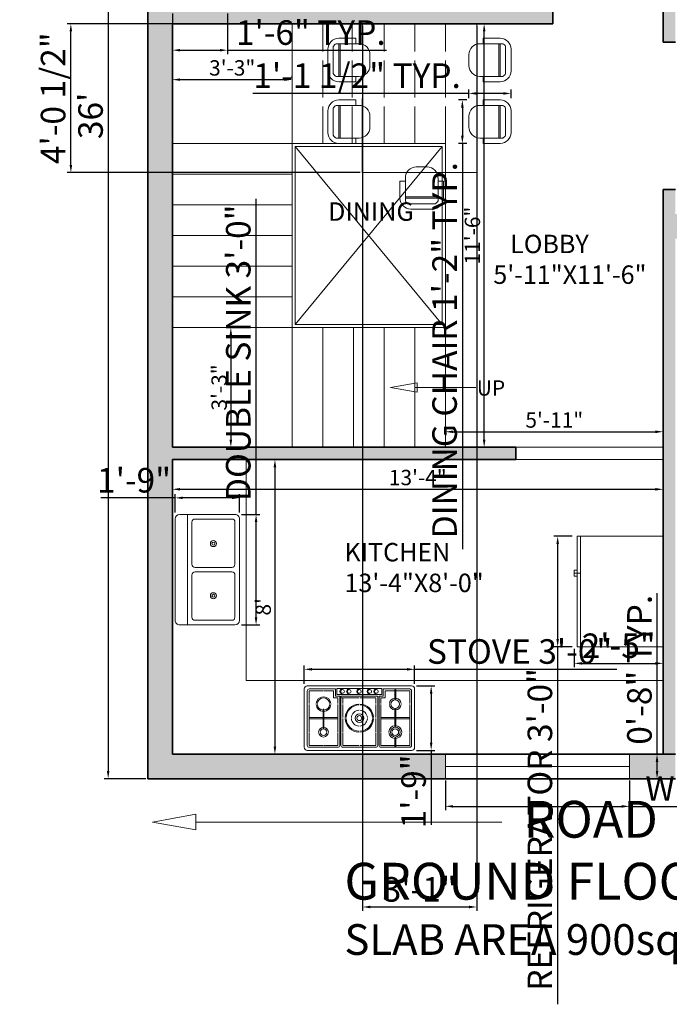
# Model space of a CAD drawing. Units: inches. Extents: x 3259 to 4981, y 1402 to 2026.
# Tile 1 of 11: x 3259 to 3471, y 1402 to 1722. Entities that reach past the tile are written whole.
import ezdxf

# ---------------------------------------------------------------- set-up
doc = ezdxf.new("R2010")
doc.units = ezdxf.units.IN
doc.linetypes.add('ACAD_ISO02W100', pattern=[15, 12, -3])
for name, color, linetype, lineweight in [('A-ANNO-DIMS', 2, 'Continuous', 13), ('A-ANNO-SYMB', 7, 'Continuous', 13), ('A-ANNO-TEXT', 7, 'Continuous', 18), ('A-ANNO-TITL', 7, 'Continuous', 25), ('A-AREA-IDEN', 7, 'Continuous', 18), ('A-DOOR', 3, 'Continuous', 18), ('A-EQPM', 8, 'Continuous', 18), ('A-FLOR-CASE', 8, 'Continuous', 18), ('A-FLOR-FIXT', 9, 'Continuous', 18), ('A-FLOR-STRS', 7, 'Continuous', 18), ('A-FLOR-STRS-OVHD', 8, 'ACAD_ISO02W100', 13), ('A-FURN', 8, 'Continuous', 13), ('A-GLAZ', 4, 'Continuous', 18), ('A-WALL', 7, 'Continuous', 35), ('A-WALL-PATT', 252, 'Continuous', 13)]:
    doc.layers.add(name, color=color, linetype=linetype, lineweight=lineweight)
doc.styles.get("Standard").update_dxf_attribs({"font": 'arial.ttf'})
doc.dimstyles.new('ISO-25', dxfattribs={"dimtxt": 8, "dimasz": 2.5, "dimexe": 1.25, "dimexo": 0.625, "dimtad": 1, "dimdec": 1, "dimlunit": 3, "dimtxsty": 'Standard', "dimcen": 2.5, "dimclrd": 4, "dimclre": 4, "dimclrt": 1, "dimadec": 0, "dimazin": 0, "dimtfac": 1, "dimtdec": 1, "dimtmove": 0, "dimatfit": 3, "dimfxl": 1, "dimarcsym": 0})

# ---------------------------------------------------------------- blocks, each defined once
blk = doc.blocks.new('STOVE')
for p, q in [((11.85, 19.7), (11.55, 19.7)), ((11.55, 16.92), (11.55, 19.7)), ((11.85, 16.92), (11.85, 19.7)), ((11.85, 16.92), (11.55, 16.92)), ((-11.85, 13.73), (-11.85, 7.62)), ((-11.85, 13.73), (-11.55, 13.73)), ((-11.55, 13.73), (-11.55, 7.62)), ((11.85, 13.23), (11.55, 13.23)), ((11.55, 13.23), (11.55, 7.57)), ((11.85, 13.23), (11.85, 7.57)), ((-11.85, 10.75), (-16.4, 10.75)), ((-11.85, 10.25), (-16.4, 10.25)), ((-7, 10.75), (-11.55, 10.75)), ((-7, 10.25), (-11.55, 10.25)), ((7, 10.75), (11.55, 10.75)), ((7, 10.25), (11.55, 10.25)), ((11.85, 10.75), (16.4, 10.75)), ((11.85, 10.25), (16.4, 10.25)), ((-11.85, 7.62), (-11.55, 7.62)), ((11.85, 7.57), (11.55, 7.57)), ((-7, 3.9), (-8.4, 3.9)), ((-7.8, 3.3), (-7.8, 1)), ((-6.4, 3.3), (-7.8, 3.3)), ((-5.4, 3.9), (-6, 3.9)), ((-5.4, 3.9), (-0.15, 3.9)), ((0.15, 3.9), (5.4, 3.9)), ((6.4, 3.3), (7.8, 3.3)), ((7, 3.9), (8.4, 3.9)), ((7.8, 3.3), (7.8, 1)), ((8.4, 3.9), (8.4, 1.6)), ((11.85, 4.28), (11.55, 4.28)), ((11.55, 4.28), (11.55, 1.3)), ((11.85, 4.28), (11.85, 1.3)), ((7.3, 2.8), (-7.3, 2.8)), ((-7.3, 2.8), (-7.3, 0.8)), ((7.3, 0.8), (-7.3, 0.8)), ((7.3, 2.8), (7.3, 0.8)), ((11.85, 1.3), (11.55, 1.3))]:
    blk.add_line(p, q)
for points in [[(-17, 21), (17, 21, -0.414214), (18, 20), (18, 1, -0.414214), (17, 0), (-17, 0, -0.414214), (-18, 1), (-18, 20, -0.414214)], [(6, 3.3), (-6, 3.3), (-6, 19.4, -0.414214), (-5.4, 20), (5.4, 20, -0.414214), (6, 19.4)]]:
    blk.add_lwpolyline(points, format="xyb", close=True)
for points in [[(-7.8, 1), (-16.4, 1, -0.414214), (-17, 1.6), (-17, 19.4, -0.414214), (-16.4, 20), (-7, 20, -0.414214), (-6.4, 19.4), (-6.4, 3.3)], [(6.4, 19.4, -0.414214), (7, 20), (16.4, 20, -0.414214), (17, 19.4), (17, 1.6, -0.414214), (16.4, 1), (7.8, 1)]]:
    blk.add_lwpolyline(points, format="xyb")
for points in [[(-16.4, 15.22), (-16.4, 19.4), (-11.85, 19.4)], [(-11.55, 19.4), (-7, 19.4), (-7, 15.22)], [(-5.4, 15.22), (-5.4, 19.4), (-0.15, 19.4)], [(0.15, 19.4), (5.4, 19.4), (5.4, 15.22)], [(6.4, 3.3), (6.4, 19.4)], [(7, 15.22), (7, 19.4), (11.55, 19.4)], [(11.85, 19.4), (16.4, 19.4), (16.4, 15.22)], [(-16.4, 6.08), (-16.4, 14.92)], [(-7, 14.92), (-7, 6.08)], [(-5.4, 10.65), (-5.4, 14.92)], [(5.4, 14.92), (5.4, 10.65)], [(7, 6.08), (7, 14.92)], [(16.4, 14.92), (16.4, 6.08)], [(-5.4, 6.08), (-5.4, 10.35)], [(5.4, 10.35), (5.4, 6.08)], [(-11.85, 1.6), (-16.4, 1.6), (-16.4, 5.77)], [(-8.4, 3.9), (-8.4, 1.6), (-11.55, 1.6)], [(-7, 5.77), (-7, 3.9)], [(-5.4, 3.9), (-5.4, 5.77)], [(5.4, 5.77), (5.4, 3.9)], [(7, 3.9), (7, 5.77)], [(16.4, 5.77), (16.4, 1.6), (11.85, 1.6)], [(11.55, 1.6), (8.4, 1.6)]]:
    blk.add_lwpolyline(points)
for centre, radius in [((-11.7, 15.07), 1.1), ((11.7, 15.07), 1.6), ((11.7, 15.07), 1.1), ((0, 10.5), 1.4), ((0, 10.5), 0.8), ((11.7, 5.93), 1.4), ((-5.49, 1.8), 0.6), ((-3.3, 1.8), 0.6), ((0, 1.8), 0.6), ((3.39, 1.8), 0.6), ((5.57, 1.8), 0.6)]:
    blk.add_circle(centre, radius)
for centre, radius, start, end in [((-11.7, 15.07), 1.6, 95.3794, 174.6206), ((-11.7, 15.07), 1.6, 5.3794, 84.6206), ((11.7, 15.07), 2.1, 94.096, 175.904), ((11.7, 15.07), 2.1, 4.096, 85.904), ((-11.7, 15.07), 1.6, 185.3794, 264.6206), ((-11.7, 15.07), 1.6, 275.3794, 354.6206), ((0, 10.5), 4.6, 91.8687, 178.1313), ((0, 10.5), 4.3, 91.9991, 178.0009), ((0, 10.5), 2.6, 93.3074, 176.6926), ((0, 10.5), 4.6, 1.8687, 88.1313), ((0, 10.5), 4.3, 1.9991, 88.0009), ((0, 10.5), 2.6, 3.3074, 86.6926), ((11.7, 15.07), 2.1, 184.096, 265.904), ((11.7, 15.07), 2.1, 274.096, 355.904), ((0, 10.5), 4.6, 181.8687, 268.1313), ((0, 10.5), 4.3, 181.9991, 268.0009), ((0, 10.5), 2.6, 183.3074, 266.6926), ((0, 10.5), 4.6, 271.8687, 358.1313), ((0, 10.5), 4.3, 271.9991, 358.0009), ((0, 10.5), 2.6, 273.3074, 356.6926), ((-11.7, 5.93), 2.4, 93.5833, 176.4167), ((-11.7, 5.93), 2, 94.3012, 175.6988), ((-11.7, 5.93), 2.4, 3.5833, 86.4167), ((-11.7, 5.93), 2, 4.3012, 85.6988), ((11.7, 5.93), 1.9, 94.5281, 175.4719), ((11.7, 5.93), 1.9, 4.5281, 85.4719), ((-11.7, 5.93), 2.4, 183.5833, 266.4167), ((-11.7, 5.93), 2, 184.3012, 265.6988), ((-11.7, 5.93), 2.4, 273.5833, 356.4167), ((-11.7, 5.93), 2, 274.3012, 355.6988), ((11.7, 5.93), 1.9, 184.5281, 265.4719), ((11.7, 5.93), 1.9, 274.5281, 355.4719), ((-5.49, 1.8), 0.846, 89.9979, 270), ((-3.3, 1.8), 0.846, 89.9979, 270), ((0, 1.8), 0.846, 89.9979, 270), ((3.39, 1.8), 0.846, 89.9979, 270), ((5.57, 1.8), 0.846, 89.9979, 270)]:
    blk.add_arc(centre, radius, start, end)
blk = doc.blocks.new('Sink-double - 36 in top')
for p, q in [((-18, -4), (18, -4)), ((-0.75, -18.5), (-0.75, -6.5)), ((0.75, -6.5), (0.75, -18.5))]:
    blk.add_line(p, q)
for points in [[(-16.5, 0), (16.5, 0)], [(-18, -19.5), (-18, -1.5)], [(18, -1.5), (18, -19.5)], [(-15.5, -5.5), (-1.75, -5.5)], [(1.75, -5.5), (15.5, -5.5)], [(-16.5, -18.5), (-16.5, -6.5)], [(16.5, -6.5), (16.5, -18.5)], [(16.5, -21), (-16.5, -21)], [(-1.75, -19.5), (-15.5, -19.5)], [(15.5, -19.5), (1.75, -19.5)]]:
    blk.add_lwpolyline(points)
for centre, radius in [((-8.5, -12.5), 1), ((-8.5, -12.5), 0.5), ((8.5, -12.5), 1), ((8.5, -12.5), 0.5)]:
    blk.add_circle(centre, radius)
for centre, radius, start, end in [((-16.5, -1.5), 1.5, 90, 180), ((16.5, -1.5), 1.5, 0, 90), ((-15.5, -6.5), 1, 90, 180), ((-1.75, -6.5), 1, 0, 90), ((1.75, -6.5), 1, 90, 180), ((15.5, -6.5), 1, 0, 90), ((-15.5, -18.5), 1, 180, 270), ((-1.75, -18.5), 1, 270, 0), ((1.75, -18.5), 1, 180, 270), ((15.5, -18.5), 1, 270, 0), ((-16.5, -19.5), 1.5, 180, 270), ((16.5, -19.5), 1.5, 270, 0)]:
    blk.add_arc(centre, radius, start, end)
blk = doc.blocks.new('Refrigerator-2 door - 36 in top')
for p, q in [((0, -26.999999), (36, -26.999999)), ((11, -27.999999), (11, -28.999999)), ((12, -26.999999), (12, -28.999999)), ((13, -28.999999), (13, -27.999999)), ((11, -28.999999), (13, -28.999999))]:
    blk.add_line(p, q)
blk.add_lwpolyline([(0, -27.999999), (0, 0), (36, 0), (36, -27.999999)], close=True)
blk = doc.blocks.new('*D22')
at = {"layer": 'A-ANNO-DIMS', "color": 0, "lineweight": -2, "transparency": 16777216}
for p, q in [((3300.54, 1907.12), (3286.97, 1907.12)), ((3288.22, 1904.62), (3288.22, 1477.62)), ((3300.54, 1475.12), (3286.97, 1475.12))]:
    blk.add_line(p, q, dxfattribs=at)
at = {"layer": 'A-ANNO-DIMS', "color": 0, "transparency": 16777216}
for points in [[(3287.81, 1904.62), (3288.64, 1904.62), (3288.22, 1907.12)], [(3287.81, 1477.62), (3288.64, 1477.62), (3288.22, 1475.12)]]:
    blk.add_solid(points, dxfattribs=at)
at = {"layer": 'Defpoints', "color": 0, "transparency": 16777216}
for p in [(3301.16, 1907.12), (3288.22, 1475.12), (3301.16, 1475.12)]:
    blk.add_point(p, dxfattribs=at)
at = {"layer": 'A-ANNO-DIMS', "color": 0, "transparency": 16777216, "insert": (3283.51, 1691.12), "char_height": 8, "attachment_point": 5, "rotation": 90}
blk.add_mtext("36'", dxfattribs=at)
blk = doc.blocks.new('*D27')
at = {"layer": 'A-ANNO-DIMS', "color": 0, "lineweight": -2, "transparency": 16777216}
for p, q in [((3469.16, 1588.81), (3469.16, 1589.43)), ((3398.16, 1587.56), (3398.16, 1586.93)), ((3400.66, 1588.18), (3466.66, 1588.18))]:
    blk.add_line(p, q, dxfattribs=at)
at = {"layer": 'A-ANNO-DIMS', "color": 0, "transparency": 16777216}
for points in [[(3400.66, 1588.6), (3400.66, 1587.76), (3398.16, 1588.18)], [(3466.66, 1588.6), (3466.66, 1587.76), (3469.16, 1588.18)]]:
    blk.add_solid(points, dxfattribs=at)
at = {"layer": 'Defpoints', "color": 0, "transparency": 16777216}
for p in [(3398.16, 1588.18), (3469.16, 1588.18), (3469.16, 1588.18)]:
    blk.add_point(p, dxfattribs=at)
at = {"layer": 'A-ANNO-DIMS', "color": 0, "transparency": 16777216, "insert": (3433.66, 1591.36), "char_height": 5, "attachment_point": 5}
blk.add_mtext('5\'-11"', dxfattribs=at)
blk = doc.blocks.new('*D28')
at = {"layer": 'A-ANNO-DIMS', "color": 0, "lineweight": -2, "transparency": 16777216}
for p, q in [((3409.02, 1721.12), (3412.05, 1721.12)), ((3410.8, 1585.62), (3410.8, 1718.62)), ((3406.72, 1583.12), (3412.05, 1583.12))]:
    blk.add_line(p, q, dxfattribs=at)
at = {"layer": 'A-ANNO-DIMS', "color": 0, "transparency": 16777216}
for points in [[(3410.39, 1718.62), (3411.22, 1718.62), (3410.8, 1721.12)], [(3410.39, 1585.62), (3411.22, 1585.62), (3410.8, 1583.12)]]:
    blk.add_solid(points, dxfattribs=at)
at = {"layer": 'Defpoints', "color": 0, "transparency": 16777216}
for p in [(3408.4, 1721.12), (3410.8, 1721.12), (3406.09, 1583.12)]:
    blk.add_point(p, dxfattribs=at)
at = {"layer": 'A-ANNO-DIMS', "color": 0, "transparency": 16777216, "insert": (3407.62, 1652.12), "char_height": 5, "attachment_point": 5, "rotation": 90}
blk.add_mtext('11\'-6"', dxfattribs=at)
blk = doc.blocks.new('*D29')
at = {"layer": 'A-ANNO-DIMS', "color": 0, "lineweight": -2, "transparency": 16777216}
for p, q in [((3309.16, 1703.55), (3309.16, 1704.17)), ((3348.16, 1703.55), (3348.16, 1704.17)), ((3311.66, 1702.92), (3345.66, 1702.92))]:
    blk.add_line(p, q, dxfattribs=at)
at = {"layer": 'A-ANNO-DIMS', "color": 0, "transparency": 16777216}
for points in [[(3311.66, 1703.34), (3311.66, 1702.51), (3309.16, 1702.92)], [(3345.66, 1703.34), (3345.66, 1702.51), (3348.16, 1702.92)]]:
    blk.add_solid(points, dxfattribs=at)
at = {"layer": 'Defpoints', "color": 0, "transparency": 16777216}
for p in [(3309.16, 1702.92), (3348.16, 1702.92), (3348.16, 1702.92)]:
    blk.add_point(p, dxfattribs=at)
at = {"layer": 'A-ANNO-DIMS', "color": 0, "transparency": 16777216, "insert": (3328.66, 1706.1), "char_height": 5, "attachment_point": 5}
blk.add_mtext('3\'-3"', dxfattribs=at)
blk = doc.blocks.new('*D30')
at = {"layer": 'A-ANNO-DIMS', "color": 0, "lineweight": -2, "transparency": 16777216}
for p, q in [((3328.84, 1622.12), (3329.47, 1622.12)), ((3328.22, 1619.62), (3328.22, 1585.62)), ((3328.84, 1583.12), (3329.47, 1583.12))]:
    blk.add_line(p, q, dxfattribs=at)
at = {"layer": 'A-ANNO-DIMS', "color": 0, "transparency": 16777216}
for points in [[(3327.8, 1619.62), (3328.63, 1619.62), (3328.22, 1622.12)], [(3327.8, 1585.62), (3328.63, 1585.62), (3328.22, 1583.12)]]:
    blk.add_solid(points, dxfattribs=at)
at = {"layer": 'Defpoints', "color": 0, "transparency": 16777216}
for p in [(3328.22, 1622.12), (3328.22, 1583.12), (3328.22, 1583.12)]:
    blk.add_point(p, dxfattribs=at)
at = {"layer": 'A-ANNO-DIMS', "color": 0, "transparency": 16777216, "insert": (3325.04, 1602.62), "char_height": 5, "attachment_point": 5, "rotation": 90}
blk.add_mtext('3\'-3"', dxfattribs=at)
blk = doc.blocks.new('*D31')
at = {"layer": 'A-ANNO-DIMS', "color": 0, "lineweight": -2, "transparency": 16777216}
for p, q in [((3309.16, 1578.49), (3309.16, 1568.19)), ((3469.16, 1578.49), (3469.16, 1568.19)), ((3311.66, 1569.44), (3466.66, 1569.44))]:
    blk.add_line(p, q, dxfattribs=at)
at = {"layer": 'A-ANNO-DIMS', "color": 0, "transparency": 16777216}
for points in [[(3311.66, 1569.85), (3311.66, 1569.02), (3309.16, 1569.44)], [(3466.66, 1569.85), (3466.66, 1569.02), (3469.16, 1569.44)]]:
    blk.add_solid(points, dxfattribs=at)
at = {"layer": 'Defpoints', "color": 0, "transparency": 16777216}
for p in [(3309.16, 1579.12), (3469.16, 1579.12), (3469.16, 1569.44)]:
    blk.add_point(p, dxfattribs=at)
at = {"layer": 'A-ANNO-DIMS', "color": 0, "transparency": 16777216, "insert": (3389.16, 1572.62), "char_height": 5, "attachment_point": 5}
blk.add_mtext('13\'-4"', dxfattribs=at)
blk = doc.blocks.new('*D32')
at = {"layer": 'A-ANNO-DIMS', "color": 0, "lineweight": -2, "transparency": 16777216}
for p, q in [((3333.79, 1579.12), (3343.84, 1579.12)), ((3342.59, 1576.62), (3342.59, 1485.62)), ((3333.79, 1483.12), (3343.84, 1483.12))]:
    blk.add_line(p, q, dxfattribs=at)
at = {"layer": 'A-ANNO-DIMS', "color": 0, "transparency": 16777216}
for points in [[(3342.17, 1576.62), (3343.01, 1576.62), (3342.59, 1579.12)], [(3342.17, 1485.62), (3343.01, 1485.62), (3342.59, 1483.12)]]:
    blk.add_solid(points, dxfattribs=at)
at = {"layer": 'Defpoints', "color": 0, "transparency": 16777216}
for p in [(3333.16, 1579.12), (3333.16, 1483.12), (3342.59, 1483.12)]:
    blk.add_point(p, dxfattribs=at)
at = {"layer": 'A-ANNO-DIMS', "color": 0, "transparency": 16777216, "insert": (3339.41, 1531.12), "char_height": 5, "attachment_point": 5, "rotation": 90}
blk.add_mtext("8'", dxfattribs=at)
blk = doc.blocks.new('CHAIR-DINING')
for p, q in [((3.55, 14.19), (9.11, 14.19)), ((9.11, 14.19), (9.11, 12.41)), ((0, 3.55), (0, 10.63)), ((1.77, 2.69), (1.77, 11.5)), ((10.19, 12.41), (2.69, 12.41)), ((3.55, 12.41), (3.55, 1.77)), ((3.99, 12.41), (3.99, 1.77)), ((13.74, 8.86), (13.74, 5.33)), ((10.19, 1.77), (2.69, 1.77)), ((9.11, 1.77), (9.11, 0)), ((9.11, 0), (3.55, 0))]:
    blk.add_line(p, q)
for centre, radius, start, end in [((3.55, 10.63), 3.55, 90, 180), ((3.55, 10.63), 1.98, 115.8945, 154.1055), ((10.19, 8.86), 3.55, 0, 90), ((3.55, 3.55), 3.55, 180, 270), ((10.19, 5.33), 3.55, 270, 0), ((3.55, 3.55), 1.98, 205.8945, 244.1055)]:
    blk.add_arc(centre, radius, start, end)
blk = doc.blocks.new('WINDOW-60x8')
for p, q in [((0, 0), (0, 8)), ((60, 0), (60, 8)), ((0, 4), (60, 4))]:
    blk.add_line(p, q)
blk = doc.blocks.new('STAIR-WELL-50x60')
for p, q in [((1, 59), (49, 1)), ((1, 1), (49, 59))]:
    blk.add_line(p, q)
for points in [[(50, 60), (0, 60), (0, 0), (50, 0)], [(49, 59), (1, 59), (1, 1), (49, 1)]]:
    blk.add_lwpolyline(points, close=True)
blk = doc.blocks.new('STAIR-DIRECTION')
blk.add_line((7.93, 1.55), (27.85, 1.55))
blk.add_lwpolyline([(0, 1.55), (8.64, 3.11), (8.64, 0)], close=True)
blk = doc.blocks.new('ROAD-DIRECTION')
blk.add_line((99.82, 2.55), (0, 2.55))
blk.add_lwpolyline([(113.98, 2.55), (99.82, 5.11), (99.82, 0)], close=True)
blk = doc.blocks.new('*D148')
at = {"layer": 'A-ANNO-DIMS', "color": 4, "lineweight": -2, "transparency": 16777216}
for p, q in [((3405.19, 1696.31), (3402.44, 1696.31)), ((3403.69, 1693.81), (3403.69, 1684.62)), ((3405.19, 1682.12), (3402.44, 1682.12)), ((3403.69, 1682.12), (3403.69, 1549.91))]:
    blk.add_line(p, q, dxfattribs=at)
at = {"layer": 'A-ANNO-DIMS', "color": 4, "transparency": 16777216}
for points in [[(3403.27, 1693.81), (3404.11, 1693.81), (3403.69, 1696.31)], [(3403.27, 1684.62), (3404.11, 1684.62), (3403.69, 1682.12)]]:
    blk.add_solid(points, dxfattribs=at)
at = {"layer": 'Defpoints', "color": 0, "transparency": 16777216}
for p in [(3405.82, 1696.31), (3403.69, 1682.12), (3405.82, 1682.12)]:
    blk.add_point(p, dxfattribs=at)
at = {"layer": 'A-ANNO-DIMS', "color": 1, "transparency": 16777216, "insert": (3398.93, 1614.76), "char_height": 8, "attachment_point": 5, "rotation": 90}
blk.add_mtext('DINING CHAIR 1\'-2" TYP.', dxfattribs=at)
blk = doc.blocks.new('*D149')
at = {"layer": 'A-ANNO-DIMS', "color": 4, "lineweight": -2, "transparency": 16777216}
for p, q in [((3405.82, 1698.43), (3335.41, 1698.43)), ((3405.82, 1696.93), (3405.82, 1699.68)), ((3417.06, 1698.43), (3408.32, 1698.43)), ((3419.56, 1696.93), (3419.56, 1699.68))]:
    blk.add_line(p, q, dxfattribs=at)
at = {"layer": 'A-ANNO-DIMS', "color": 4, "transparency": 16777216}
for points in [[(3408.32, 1698.85), (3408.32, 1698.02), (3405.82, 1698.43)], [(3417.06, 1698.85), (3417.06, 1698.02), (3419.56, 1698.43)]]:
    blk.add_solid(points, dxfattribs=at)
at = {"layer": 'Defpoints', "color": 0, "transparency": 16777216}
for p in [(3405.82, 1698.43), (3405.82, 1696.31), (3419.56, 1696.31)]:
    blk.add_point(p, dxfattribs=at)
at = {"layer": 'A-ANNO-DIMS', "color": 1, "transparency": 16777216, "insert": (3369.37, 1703.19), "char_height": 8, "attachment_point": 5}
blk.add_mtext('1\'-1 1/2" TYP.', dxfattribs=at)
blk = doc.blocks.new('*D165')
at = {"layer": 'A-ANNO-DIMS', "color": 4, "lineweight": -2, "transparency": 16777216}
for p, q in [((3309.16, 1724.49), (3309.16, 1711.27)), ((3327.16, 1724.49), (3327.16, 1711.27)), ((3311.66, 1712.52), (3324.66, 1712.52)), ((3327.16, 1712.52), (3378.93, 1712.52))]:
    blk.add_line(p, q, dxfattribs=at)
at = {"layer": 'A-ANNO-DIMS', "color": 4, "transparency": 16777216}
for points in [[(3311.66, 1712.93), (3311.66, 1712.1), (3309.16, 1712.52)], [(3324.66, 1712.93), (3324.66, 1712.1), (3327.16, 1712.52)]]:
    blk.add_solid(points, dxfattribs=at)
at = {"layer": 'Defpoints', "color": 0, "transparency": 16777216}
for p in [(3309.16, 1725.12), (3327.16, 1725.12), (3327.16, 1712.52)]:
    blk.add_point(p, dxfattribs=at)
at = {"layer": 'A-ANNO-DIMS', "color": 1, "transparency": 16777216, "insert": (3354.29, 1717.23), "char_height": 8, "attachment_point": 5}
blk.add_mtext('1\'-6" TYP.', dxfattribs=at)
blk = doc.blocks.new('*D174')
at = {"layer": 'A-ANNO-DIMS', "color": 4, "lineweight": -2, "transparency": 16777216}
for p, q in [((3398.16, 1474.49), (3398.16, 1464.87)), ((3458.16, 1474.49), (3458.16, 1464.87)), ((3400.66, 1466.12), (3455.66, 1466.12)), ((3458.16, 1466.12), (3563.15, 1466.12))]:
    blk.add_line(p, q, dxfattribs=at)
at = {"layer": 'A-ANNO-DIMS', "color": 4, "transparency": 16777216}
for points in [[(3400.66, 1466.53), (3400.66, 1465.7), (3398.16, 1466.12)], [(3455.66, 1466.53), (3455.66, 1465.7), (3458.16, 1466.12)]]:
    blk.add_solid(points, dxfattribs=at)
at = {"layer": 'Defpoints', "color": 0, "transparency": 16777216}
for p in [(3398.16, 1475.12), (3458.16, 1475.12), (3458.16, 1466.12)]:
    blk.add_point(p, dxfattribs=at)
at = {"layer": 'A-ANNO-DIMS', "color": 1, "transparency": 16777216, "insert": (3511.91, 1470.88), "char_height": 8, "attachment_point": 5}
blk.add_mtext('WINDOW 5\'-0" TYP.', dxfattribs=at)
blk = doc.blocks.new('*D175')
at = {"layer": 'A-ANNO-DIMS', "color": 4, "lineweight": -2, "transparency": 16777216}
for p, q in [((3467.16, 1483.12), (3467.16, 1535.63)), ((3458.79, 1483.12), (3468.41, 1483.12)), ((3467.16, 1477.62), (3467.16, 1480.62)), ((3458.79, 1475.12), (3468.41, 1475.12))]:
    blk.add_line(p, q, dxfattribs=at)
at = {"layer": 'A-ANNO-DIMS', "color": 4, "transparency": 16777216}
for points in [[(3466.75, 1480.62), (3467.58, 1480.62), (3467.16, 1483.12)], [(3466.75, 1477.62), (3467.58, 1477.62), (3467.16, 1475.12)]]:
    blk.add_solid(points, dxfattribs=at)
at = {"layer": 'Defpoints', "color": 0, "transparency": 16777216}
for p in [(3458.16, 1483.12), (3467.16, 1483.12), (3458.16, 1475.12)]:
    blk.add_point(p, dxfattribs=at)
at = {"layer": 'A-ANNO-DIMS', "color": 1, "transparency": 16777216, "insert": (3462.45, 1510.62), "char_height": 8, "attachment_point": 5, "rotation": 90}
blk.add_mtext('0\'-8" TYP.', dxfattribs=at)
blk = doc.blocks.new('*D180')
at = {"layer": 'A-ANNO-DIMS', "color": 4, "lineweight": -2, "transparency": 16777216}
for p, q in [((3352.12, 1505.99), (3352.12, 1512.02)), ((3388.12, 1505.99), (3388.12, 1512.02)), ((3354.62, 1510.77), (3385.62, 1510.77)), ((3388.12, 1510.77), (3454.09, 1510.77))]:
    blk.add_line(p, q, dxfattribs=at)
at = {"layer": 'A-ANNO-DIMS', "color": 4, "transparency": 16777216}
for points in [[(3354.62, 1511.19), (3354.62, 1510.35), (3352.12, 1510.77)], [(3385.62, 1511.19), (3385.62, 1510.35), (3388.12, 1510.77)]]:
    blk.add_solid(points, dxfattribs=at)
at = {"layer": 'Defpoints', "color": 0, "transparency": 16777216}
for p in [(3388.12, 1510.77), (3352.12, 1505.37), (3388.12, 1505.37)]:
    blk.add_point(p, dxfattribs=at)
at = {"layer": 'A-ANNO-DIMS', "color": 1, "transparency": 16777216, "insert": (3422.36, 1515.54), "char_height": 8, "attachment_point": 5}
blk.add_mtext('STOVE 3\'-0"', dxfattribs=at)
blk = doc.blocks.new('*D181')
at = {"layer": 'A-ANNO-DIMS', "color": 4, "lineweight": -2, "transparency": 16777216}
for p, q in [((3388.75, 1505.37), (3394.77, 1505.37)), ((3393.52, 1502.87), (3393.52, 1486.87)), ((3388.75, 1484.37), (3394.77, 1484.37)), ((3393.52, 1484.37), (3393.52, 1460.11))]:
    blk.add_line(p, q, dxfattribs=at)
at = {"layer": 'A-ANNO-DIMS', "color": 4, "transparency": 16777216}
for points in [[(3393.11, 1502.87), (3393.94, 1502.87), (3393.52, 1505.37)], [(3393.11, 1486.87), (3393.94, 1486.87), (3393.52, 1484.37)]]:
    blk.add_solid(points, dxfattribs=at)
at = {"layer": 'Defpoints', "color": 0, "transparency": 16777216}
for p in [(3388.12, 1505.37), (3388.12, 1484.37), (3393.52, 1484.37)]:
    blk.add_point(p, dxfattribs=at)
at = {"layer": 'A-ANNO-DIMS', "color": 1, "transparency": 16777216, "insert": (3388.81, 1470.99), "char_height": 8, "attachment_point": 5, "rotation": 90}
blk.add_mtext('1\'-9"', dxfattribs=at)
blk = doc.blocks.new('*D182')
at = {"layer": 'A-ANNO-DIMS', "color": 4, "lineweight": -2, "transparency": 16777216}
for p, q in [((3336.44, 1561.24), (3336.44, 1664.12)), ((3331.66, 1561.24), (3337.69, 1561.24)), ((3336.44, 1527.74), (3336.44, 1558.74)), ((3331.66, 1525.24), (3337.69, 1525.24))]:
    blk.add_line(p, q, dxfattribs=at)
at = {"layer": 'A-ANNO-DIMS', "color": 4, "transparency": 16777216}
for points in [[(3336.02, 1558.74), (3336.86, 1558.74), (3336.44, 1561.24)], [(3336.02, 1527.74), (3336.86, 1527.74), (3336.44, 1525.24)]]:
    blk.add_solid(points, dxfattribs=at)
at = {"layer": 'Defpoints', "color": 0, "transparency": 16777216}
for p in [(3331.04, 1561.24), (3336.44, 1561.24), (3331.04, 1525.24)]:
    blk.add_point(p, dxfattribs=at)
at = {"layer": 'A-ANNO-DIMS', "color": 1, "transparency": 16777216, "insert": (3331.67, 1613.93), "char_height": 8, "attachment_point": 5, "rotation": 90}
blk.add_mtext('DOUBLE SINK 3\'-0"', dxfattribs=at)
blk = doc.blocks.new('*D183')
at = {"layer": 'A-ANNO-DIMS', "color": 4, "lineweight": -2, "transparency": 16777216}
for p, q in [((3310.04, 1566.64), (3285.78, 1566.64)), ((3310.04, 1561.87), (3310.04, 1567.89)), ((3328.54, 1566.64), (3312.54, 1566.64)), ((3331.04, 1561.87), (3331.04, 1567.89))]:
    blk.add_line(p, q, dxfattribs=at)
at = {"layer": 'A-ANNO-DIMS', "color": 4, "transparency": 16777216}
for points in [[(3312.54, 1567.06), (3312.54, 1566.23), (3310.04, 1566.64)], [(3328.54, 1567.06), (3328.54, 1566.23), (3331.04, 1566.64)]]:
    blk.add_solid(points, dxfattribs=at)
at = {"layer": 'Defpoints', "color": 0, "transparency": 16777216}
for p in [(3310.04, 1566.64), (3310.04, 1561.24), (3331.04, 1561.24)]:
    blk.add_point(p, dxfattribs=at)
at = {"layer": 'A-ANNO-DIMS', "color": 1, "transparency": 16777216, "insert": (3296.66, 1571.35), "char_height": 8, "attachment_point": 5}
blk.add_mtext('1\'-9"', dxfattribs=at)
blk = doc.blocks.new('*D184')
at = {"layer": 'A-ANNO-DIMS', "color": 4, "lineweight": -2, "transparency": 16777216}
for p, q in [((3439.54, 1554.11), (3433.51, 1554.11)), ((3434.76, 1551.61), (3434.76, 1520.61)), ((3439.54, 1518.11), (3433.51, 1518.11)), ((3434.76, 1518.11), (3434.76, 1401.61))]:
    blk.add_line(p, q, dxfattribs=at)
at = {"layer": 'A-ANNO-DIMS', "color": 4, "transparency": 16777216}
for points in [[(3434.35, 1551.61), (3435.18, 1551.61), (3434.76, 1554.11)], [(3434.35, 1520.61), (3435.18, 1520.61), (3434.76, 1518.11)]]:
    blk.add_solid(points, dxfattribs=at)
at = {"layer": 'Defpoints', "color": 0, "transparency": 16777216}
for p in [(3440.16, 1554.11), (3434.76, 1518.11), (3440.16, 1518.11)]:
    blk.add_point(p, dxfattribs=at)
at = {"layer": 'A-ANNO-DIMS', "color": 1, "transparency": 16777216, "insert": (3430, 1458.61), "char_height": 8, "attachment_point": 5, "rotation": 90}
blk.add_mtext('REFRIGERATOR 3\'-0"', dxfattribs=at)
blk = doc.blocks.new('*D185')
at = {"layer": 'A-ANNO-DIMS', "color": 4, "lineweight": -2, "transparency": 16777216}
for p, q in [((3440.16, 1517.48), (3440.16, 1511.46)), ((3469.16, 1517.48), (3469.16, 1511.46)), ((3442.66, 1512.71), (3466.66, 1512.71))]:
    blk.add_line(p, q, dxfattribs=at)
at = {"layer": 'A-ANNO-DIMS', "color": 4, "transparency": 16777216}
for points in [[(3442.66, 1513.12), (3442.66, 1512.29), (3440.16, 1512.71)], [(3466.66, 1513.12), (3466.66, 1512.29), (3469.16, 1512.71)]]:
    blk.add_solid(points, dxfattribs=at)
at = {"layer": 'Defpoints', "color": 0, "transparency": 16777216}
for p in [(3440.16, 1518.11), (3469.16, 1518.11), (3469.16, 1512.71)]:
    blk.add_point(p, dxfattribs=at)
at = {"layer": 'A-ANNO-DIMS', "color": 1, "transparency": 16777216, "insert": (3454.66, 1517.42), "char_height": 8, "attachment_point": 5}
blk.add_mtext('2\'-5"', dxfattribs=at)
blk = doc.blocks.new('*D190')
at = {"layer": 'A-ANNO-DIMS', "color": 4, "lineweight": -2, "transparency": 16777216}
for p, q in [((3371.16, 1720.49), (3371.16, 1432.07)), ((3408.4, 1720.49), (3408.4, 1432.07)), ((3373.66, 1433.32), (3405.9, 1433.32))]:
    blk.add_line(p, q, dxfattribs=at)
at = {"layer": 'A-ANNO-DIMS', "color": 4, "transparency": 16777216}
for points in [[(3373.66, 1433.74), (3373.66, 1432.9), (3371.16, 1433.32)], [(3405.9, 1433.74), (3405.9, 1432.9), (3408.4, 1433.32)]]:
    blk.add_solid(points, dxfattribs=at)
at = {"layer": 'Defpoints', "color": 0, "transparency": 16777216}
for p in [(3371.16, 1721.12), (3408.4, 1721.12), (3408.4, 1433.32)]:
    blk.add_point(p, dxfattribs=at)
at = {"layer": 'A-ANNO-DIMS', "color": 1, "transparency": 16777216, "insert": (3389.78, 1438.03), "char_height": 8, "attachment_point": 5}
blk.add_mtext('3\'-1"', dxfattribs=at)
blk = doc.blocks.new('*D191')
at = {"layer": 'A-ANNO-DIMS', "color": 4, "lineweight": -2, "transparency": 16777216}
for p, q in [((3370.54, 1721.12), (3274.81, 1721.12)), ((3276.06, 1675.12), (3276.06, 1718.62)), ((3370.37, 1672.62), (3274.81, 1672.62))]:
    blk.add_line(p, q, dxfattribs=at)
at = {"layer": 'A-ANNO-DIMS', "color": 4, "transparency": 16777216}
for points in [[(3275.65, 1718.62), (3276.48, 1718.62), (3276.06, 1721.12)], [(3275.65, 1675.12), (3276.48, 1675.12), (3276.06, 1672.62)]]:
    blk.add_solid(points, dxfattribs=at)
at = {"layer": 'Defpoints', "color": 0, "transparency": 16777216}
for p in [(3276.06, 1721.12), (3371.16, 1721.12), (3370.99, 1672.62)]:
    blk.add_point(p, dxfattribs=at)
at = {"layer": 'A-ANNO-DIMS', "color": 1, "transparency": 16777216, "insert": (3271.3, 1696.87), "char_height": 8, "attachment_point": 5, "rotation": 90}
blk.add_mtext('4\'-0 1/2"', dxfattribs=at)

msp = doc.modelspace()

# ---------------------------------------------------------------- hatches: boundary and pattern name
at = {"layer": 'A-WALL-PATT'}
h = msp.add_hatch(color=256, dxfattribs=at)
h.dxf.hatch_style = 1
h.paths.add_polyline_path([(3601.16, 1907.12), (3301.16, 1907.12), (3301.16, 1475.12), (3398.16, 1475.12), (3398.16, 1483.12), (3309.16, 1483.12), (3309.16, 1579.12), (3421.16, 1579.12), (3421.16, 1583.12), (3309.16, 1583.12), (3309.16, 1721.12), (3433.16, 1721.12), (3433.16, 1725.12), (3309.16, 1725.12), (3309.16, 1899.12), (3345.16, 1899.12), (3345.16, 1881.12), (3349.16, 1881.12), (3349.16, 1899.12), (3429.16, 1899.12), (3429.16, 1887.12), (3433.16, 1887.12), (3433.16, 1899.12), (3505.16, 1899.12), (3505.16, 1887.12), (3509.16, 1887.12), (3509.16, 1899.12), (3593.16, 1899.12), (3593.16, 1851.12), (3539.16, 1851.12), (3539.16, 1847.12), (3593.16, 1847.12), (3593.16, 1659.12), (3587.16, 1659.12), (3587.16, 1651.12), (3593.16, 1651.12), (3593.16, 1475.12), (3601.16, 1475.12)])
h.paths.add_polyline_path([(3433.16, 1863.12), (3429.16, 1863.12), (3429.16, 1851.12), (3345.16, 1851.12), (3345.16, 1847.12), (3382.99, 1847.12), (3382.99, 1847.13), (3383.04, 1847.13), (3383.04, 1847.12), (3387.07, 1847.12), (3387.07, 1847.12), (3387.11, 1847.12), (3433.16, 1847.12)], flags=17)
h.paths.add_polyline_path([(3509.16, 1863.12), (3505.16, 1863.12), (3505.16, 1847.12), (3509.16, 1847.12)], flags=17)
h.paths.add_polyline_path([(3473.16, 1851.12), (3469.16, 1851.12), (3469.16, 1715.12), (3473.16, 1715.12), (3473.16, 1777.43), (3473.16, 1777.43), (3473.16, 1777.47), (3473.16, 1777.47), (3473.16, 1781.5), (3473.16, 1781.5), (3473.16, 1781.55)], flags=17)
h.paths.add_polyline_path([(3491.16, 1659.12), (3473.16, 1659.12), (3473.16, 1667.12), (3469.16, 1667.12), (3469.16, 1483.12), (3473.16, 1483.12), (3473.16, 1651.12), (3491.16, 1651.12)], flags=17)
h.paths.add_polyline_path([(3551.16, 1659.12), (3539.16, 1659.12), (3539.16, 1651.12), (3551.16, 1651.12)], flags=17)
h.paths.add_polyline_path([(3473.16, 1483.12), (3458.16, 1483.12), (3458.16, 1475.12), (3473.16, 1475.12)], flags=17)

# ---------------------------------------------------------------- linework, layer by layer
at = {"layer": 'A-DOOR'}
for p, q in [((3421.16, 1583.12), (3469.16, 1583.12)), ((3421.16, 1579.12), (3469.16, 1579.12))]:
    msp.add_line(p, q, dxfattribs=at)
at = {"layer": 'A-FLOR-CASE'}
for p, q in [((3333.16, 1507.12), (3333.16, 1579.12)), ((3469.16, 1507.12), (3333.16, 1507.12))]:
    msp.add_line(p, q, dxfattribs=at)
at = {"layer": 'A-FLOR-STRS'}
for p, q in [((3348.16, 1583.12), (3348.16, 1721.12)), ((3309.16, 1682.12), (3398.16, 1682.12)), ((3309.16, 1672.12), (3348.16, 1672.12)), ((3309.16, 1662.12), (3348.16, 1662.12)), ((3309.16, 1652.12), (3348.16, 1652.12)), ((3309.16, 1642.12), (3348.16, 1642.12)), ((3309.16, 1632.12), (3348.16, 1632.12)), ((3398.16, 1622.12), (3309.16, 1622.12)), ((3358.16, 1583.12), (3358.16, 1622.12)), ((3368.16, 1583.12), (3368.16, 1622.12)), ((3378.16, 1583.12), (3378.16, 1622.12)), ((3388.16, 1583.12), (3388.16, 1622.12)), ((3398.16, 1583.12), (3398.16, 1622.12))]:
    msp.add_line(p, q, dxfattribs=at)
at = {"layer": 'A-FLOR-STRS-OVHD'}
for p, q in [((3358.16, 1682.12), (3358.16, 1721.12)), ((3367.79, 1682.12), (3367.79, 1721.12)), ((3378.16, 1682.12), (3378.16, 1721.12)), ((3388.16, 1682.12), (3388.16, 1721.12)), ((3398.16, 1682.12), (3398.16, 1721.12))]:
    msp.add_line(p, q, dxfattribs=at)
at = {"layer": 'A-FURN'}
for p, q in [((3370.99, 1672.62), (3371.16, 1721.12)), ((3408.4, 1672.62), (3408.4, 1721.12)), ((3370.99, 1672.62), (3408.4, 1672.62))]:
    msp.add_line(p, q, dxfattribs=at)
at = {"layer": 'A-WALL'}
for p, q in [((3469.16, 1715.12), (3469.16, 1851.12)), ((3433.16, 1721.12), (3433.16, 1725.12)), ((3309.16, 1721.12), (3433.16, 1721.12)), ((3309.16, 1583.12), (3309.16, 1721.12)), ((3469.16, 1715.12), (3473.16, 1715.12)), ((3469.16, 1483.12), (3469.16, 1667.12)), ((3469.16, 1667.12), (3473.16, 1667.12)), ((3421.16, 1583.12), (3309.16, 1583.12)), ((3421.16, 1579.12), (3421.16, 1583.12)), ((3309.16, 1483.12), (3309.16, 1579.12)), ((3421.16, 1579.12), (3309.16, 1579.12)), ((3473.16, 1483.12), (3309.16, 1483.12))]:
    msp.add_line(p, q, dxfattribs=at)
msp.add_lwpolyline([(3473.16, 1475.12), (3301.16, 1475.12), (3301.16, 1907.12), (3601.16, 1907.12), (3601.16, 1475.12), (3593.16, 1475.12)], dxfattribs=at)

# ---------------------------------------------------------------- block references
at = {"layer": 'A-ANNO-SYMB'}
msp.add_blockref('STAIR-DIRECTION', (3380.28, 1601.06), dxfattribs=at)
at = {"layer": 'A-ANNO-SYMB', "rotation": 180}
msp.add_blockref('ROAD-DIRECTION', (3416.61, 1463.53), dxfattribs=at)
at = {"layer": 'A-EQPM', "rotation": 270}
msp.add_blockref('Refrigerator-2 door - 36 in top', (3469.16, 1554.11), dxfattribs=at)
at = {"layer": 'A-EQPM', "xscale": -1, "rotation": 180}
msp.add_blockref('STOVE', (3370.12, 1505.37), dxfattribs=at)
at = {"layer": 'A-FLOR-FIXT', "rotation": 89.99999999999999}
msp.add_blockref('Sink-double - 36 in top', (3310.04, 1543.24), dxfattribs=at)
at = {"layer": 'A-FLOR-STRS'}
msp.add_blockref('STAIR-WELL-50x60', (3348.16, 1622.12), dxfattribs=at)
at = {"layer": 'A-FURN'}
for p in [(3359.83, 1702.21), (3359.83, 1682.12)]:
    msp.add_blockref('CHAIR-DINING', p, dxfattribs=at)
for p, rotation in [((3419.56, 1716.4), 180), ((3419.56, 1696.31), 180), ((3397.53, 1660.72), 90)]:
    msp.add_blockref('CHAIR-DINING', p, dxfattribs=dict(at, rotation=rotation))
at = {"layer": 'A-GLAZ'}
msp.add_blockref('WINDOW-60x8', (3398.16, 1475.12), dxfattribs=at)

# ---------------------------------------------------------------- texts
at = {"layer": 'A-ANNO-SYMB', "insert": (3417.64, 1604.94), "char_height": 5, "attachment_point": 3}
msp.add_mtext_dynamic_manual_height_columns('UP', width=10.7355, gutter_width=12.5, heights=[0], dxfattribs=at)
at = {"layer": 'A-ANNO-TEXT', "insert": (3416.34, 1467.9), "char_height": 12, "attachment_point": 1}
msp.add_mtext_dynamic_manual_height_columns('  ROAD', width=86.9528, gutter_width=12.5, heights=[0], dxfattribs=at)
at = {"layer": 'A-ANNO-TITL', "insert": (3365.25, 1447.72), "char_height": 12, "attachment_point": 1}
msp.add_mtext_dynamic_manual_height_columns('GROUND FLOOR PLAN\\P{\\H0.83333x;SLAB AREA 900sq.ft.}', width=298.7081, gutter_width=12.5, heights=[0], dxfattribs=at)
at = {"layer": 'A-AREA-IDEN', "char_height": 6, "attachment_point": 1}
for s, insert in [('DINING', (3359.93, 1662.93)), ('   LOBBY\\P5\'-11"X11\'-6"', (3413.78, 1652.38)), ('KITCHEN\\P13\'-4"X8\'-0"', (3365.25, 1551.94))]:
    msp.add_mtext_dynamic_manual_height_columns(s, width=127.3061, gutter_width=12.5, heights=[0], dxfattribs=dict(at, insert=insert))

# ---------------------------------------------------------------- dimensions: what is measured, and where the dimension line sits
at = {"layer": 'A-ANNO-DIMS'}
for base, p1, p2, angle, override, picture, middle in [((3288.22, 1475.12), (3301.16, 1907.12), (3301.16, 1475.12), 90, {"dimclrd": 0, "dimclre": 0, "dimclrt": 0}, '*D22', (3283.51, 1691.12)), ((3276.06, 1721.12), (3370.99, 1672.62), (3371.16, 1721.12), 90, {"dimdec": 1, "dimlfac": 1, "dimrnd": 0, "dimzin": 1, "dimdsep": 46, "dimlunit": 4, "dimfrac": 2}, '*D191', (3271.3, 1696.87)), ((3410.8, 1721.12), (3406.09, 1583.12), (3408.4, 1721.12), 90, {"dimtxt": 5, "dimclrd": 0, "dimclre": 0, "dimclrt": 0}, '*D28', (3407.62, 1652.12)), ((3328.22, 1583.12), (3328.22, 1622.12), (3328.22, 1583.12), 90, {"dimtxt": 5, "dimclrd": 0, "dimclre": 0, "dimclrt": 0}, '*D30', (3325.04, 1602.62)), ((3342.59, 1483.12), (3333.16, 1579.12), (3333.16, 1483.12), 90, {"dimtxt": 5, "dimclrd": 0, "dimclre": 0, "dimclrt": 0}, '*D32', (3339.41, 1531.12)), ((3310.04, 1566.64), (3331.04, 1561.24), (3310.04, 1561.24), 180, {"dimdec": 1, "dimlfac": 1, "dimrnd": 0, "dimzin": 1, "dimdsep": 46, "dimlunit": 4, "dimfrac": 2}, '*D183', (3296.66, 1571.35)), ((3393.52, 1484.37), (3388.12, 1505.37), (3388.12, 1484.37), 270, {"dimdec": 1, "dimlfac": 1, "dimrnd": 0, "dimzin": 1, "dimdsep": 46, "dimlunit": 4, "dimfrac": 2}, '*D181', (3388.81, 1470.99))]:
    dim = msp.add_linear_dim(base=base, p1=p1, p2=p2, angle=angle, dimstyle='ISO-25', override=override, dxfattribs=at)
    dim.commit()
    dim.dimension.update_dxf_attribs({"geometry": picture, "text_midpoint": middle})
for base, p1, p2, text, picture, middle in [((3327.16, 1712.52), (3309.16, 1725.12), (3327.16, 1725.12), '<> TYP.', '*D165', (3354.29, 1717.23)), ((3388.12, 1510.77), (3352.12, 1505.37), (3388.12, 1505.37), 'STOVE <>', '*D180', (3422.36, 1515.54)), ((3458.16, 1466.12), (3398.16, 1475.12), (3458.16, 1475.12), 'WINDOW <> TYP.', '*D174', (3511.91, 1470.88))]:
    dim = msp.add_linear_dim(base=base, p1=p1, p2=p2, text=text, dimstyle='ISO-25', override={"dimdec": 1, "dimlfac": 1, "dimrnd": 0, "dimzin": 1, "dimdsep": 46, "dimlunit": 4, "dimfrac": 2}, dxfattribs=at)
    dim.commit()
    dim.dimension.update_dxf_attribs({"geometry": picture, "text_midpoint": middle})
for base, p1, p2, angle, text, picture, middle in [((3405.82, 1698.43), (3419.56, 1696.31), (3405.82, 1696.31), 180, '<> TYP.', '*D149', (3369.37, 1703.19)), ((3403.69, 1682.12), (3405.82, 1696.31), (3405.82, 1682.12), 270, 'DINING CHAIR <> TYP.', '*D148', (3398.93, 1614.76)), ((3336.44, 1561.24), (3331.04, 1525.24), (3331.04, 1561.24), 90, 'DOUBLE SINK <>', '*D182', (3331.67, 1613.93)), ((3434.76, 1518.11), (3440.16, 1554.11), (3440.16, 1518.11), 270, 'REFRIGERATOR <>', '*D184', (3430, 1458.61)), ((3467.16, 1483.12), (3458.16, 1475.12), (3458.16, 1483.12), 90, '<> TYP.', '*D175', (3462.45, 1510.62))]:
    dim = msp.add_linear_dim(base=base, p1=p1, p2=p2, angle=angle, text=text, dimstyle='ISO-25', override={"dimdec": 1, "dimlfac": 1, "dimrnd": 0, "dimzin": 1, "dimdsep": 46, "dimlunit": 4, "dimfrac": 2}, dxfattribs=at)
    dim.commit()
    dim.dimension.update_dxf_attribs({"geometry": picture, "text_midpoint": middle})
for base, p1, p2, override, picture, middle in [((3408.4, 1433.32), (3371.16, 1721.12), (3408.4, 1721.12), {"dimdec": 1, "dimlfac": 1, "dimrnd": 0, "dimzin": 1, "dimdsep": 46, "dimlunit": 4, "dimfrac": 2}, '*D190', (3389.78, 1438.03)), ((3348.16, 1702.92), (3309.16, 1702.92), (3348.16, 1702.92), {"dimtxt": 5, "dimclrd": 0, "dimclre": 0, "dimclrt": 0}, '*D29', (3328.66, 1706.1)), ((3469.16, 1588.18), (3398.16, 1588.18), (3469.16, 1588.18), {"dimtxt": 5, "dimclrd": 0, "dimclre": 0, "dimclrt": 0}, '*D27', (3433.66, 1591.36)), ((3469.16, 1569.44), (3309.16, 1579.12), (3469.16, 1579.12), {"dimtxt": 5, "dimclrd": 0, "dimclre": 0, "dimclrt": 0}, '*D31', (3389.16, 1572.62)), ((3469.16, 1512.71), (3440.16, 1518.11), (3469.16, 1518.11), {"dimdec": 1, "dimlfac": 1, "dimrnd": 0, "dimzin": 1, "dimdsep": 46, "dimlunit": 4, "dimfrac": 2}, '*D185', (3454.66, 1517.42))]:
    dim = msp.add_linear_dim(base=base, p1=p1, p2=p2, dimstyle='ISO-25', override=override, dxfattribs=at)
    dim.commit()
    dim.dimension.update_dxf_attribs({"geometry": picture, "text_midpoint": middle})

doc.saveas('drawing.dxf')
